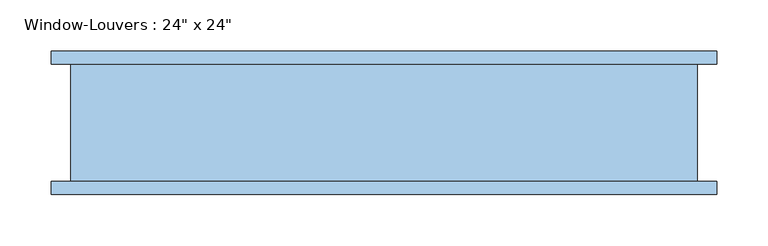
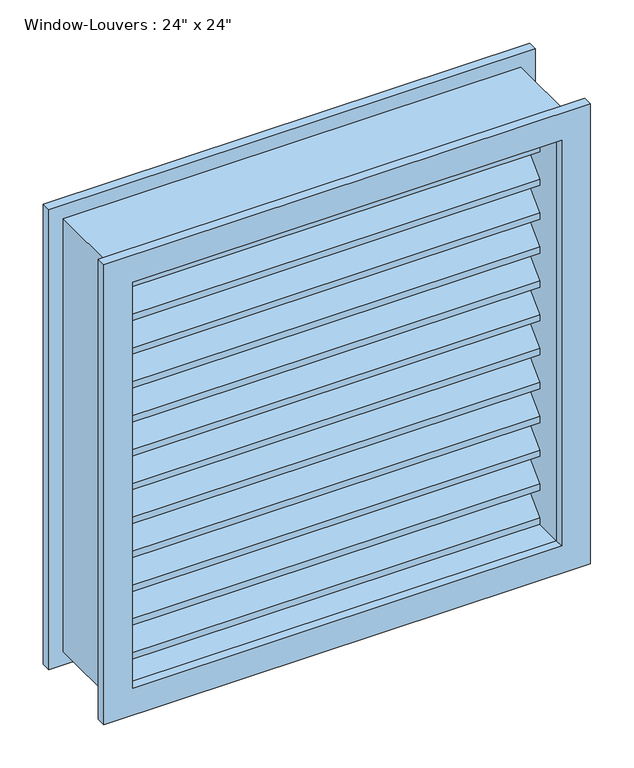
"""IFC4 building model written with IfcOpenShell, lengths in millimetres: window geometry."""

from ifc_helpers import new_model, si_unit, frame, origin, place, context, project, spatial, polyline, outline, extrude, source, transform, mapped, element, save


def window_d39e7ecb(model_context):
    return source(origin(), model_context, "Body", "SweptSolid", [
        extrude(outline(polyline([(50.8, 1419.1754778), (50.8, 1410.1952217), (12.7, 1448.2952217), (-25.4, 1410.1952217), (-25.4, 1419.1754778), (12.7, 1457.2754778), (50.8, 1419.1754778)])), frame((-285.75, 0.0, 0.0), z_axis=(1.0, 0.0, 0.0), x_axis=(0.0, 1.0, 0.0)), (0.0, 0.0, 1.0), 571.5),
        extrude(outline(polyline([(50.8, 1371.5009557), (50.8, 1362.5206995), (12.7, 1400.6206995), (-25.4, 1362.5206995), (-25.4, 1371.5009557), (12.7, 1409.6009557), (50.8, 1371.5009557)])), frame((-285.75, 0.0, 0.0), z_axis=(1.0, 0.0, 0.0), x_axis=(0.0, 1.0, 0.0)), (0.0, 0.0, 1.0), 571.5),
        extrude(outline(polyline([(50.8, 1323.8264335), (50.8, 1314.8461774), (12.7, 1352.9461774), (-25.4, 1314.8461774), (-25.4, 1323.8264335), (12.7, 1361.9264335), (50.8, 1323.8264335)])), frame((-285.75, 0.0, 0.0), z_axis=(1.0, 0.0, 0.0), x_axis=(0.0, 1.0, 0.0)), (0.0, 0.0, 1.0), 571.5),
        extrude(outline(polyline([(50.8, 1276.1519113), (50.8, 1267.1716552), (12.7, 1305.2716552), (-25.4, 1267.1716552), (-25.4, 1276.1519113), (12.7, 1314.2519113), (50.8, 1276.1519113)])), frame((-285.75, 0.0, 0.0), z_axis=(1.0, 0.0, 0.0), x_axis=(0.0, 1.0, 0.0)), (0.0, 0.0, 1.0), 571.5),
        extrude(outline(polyline([(50.8, 1228.4773891), (50.8, 1219.497133), (12.7, 1257.597133), (-25.4, 1219.497133), (-25.4, 1228.4773891), (12.7, 1266.5773891), (50.8, 1228.4773891)])), frame((-285.75, 0.0, 0.0), z_axis=(1.0, 0.0, 0.0), x_axis=(0.0, 1.0, 0.0)), (0.0, 0.0, 1.0), 571.5),
        extrude(outline(polyline([(50.8, 1180.802867), (50.8, 1171.8226109), (12.7, 1209.9226109), (-25.4, 1171.8226109), (-25.4, 1180.802867), (12.7, 1218.902867), (50.8, 1180.802867)])), frame((-285.75, 0.0, 0.0), z_axis=(1.0, 0.0, 0.0), x_axis=(0.0, 1.0, 0.0)), (0.0, 0.0, 1.0), 571.5),
        extrude(outline(polyline([(50.8, 1133.1283448), (50.8, 1124.1480887), (12.7, 1162.2480887), (-25.4, 1124.1480887), (-25.4, 1133.1283448), (12.7, 1171.2283448), (50.8, 1133.1283448)])), frame((-285.75, 0.0, 0.0), z_axis=(1.0, 0.0, 0.0), x_axis=(0.0, 1.0, 0.0)), (0.0, 0.0, 1.0), 571.5),
        extrude(outline(polyline([(50.8, 1085.4538226), (50.8, 1076.4735665), (12.7, 1114.5735665), (-25.4, 1076.4735665), (-25.4, 1085.4538226), (12.7, 1123.5538226), (50.8, 1085.4538226)])), frame((-285.75, 0.0, 0.0), z_axis=(1.0, 0.0, 0.0), x_axis=(0.0, 1.0, 0.0)), (0.0, 0.0, 1.0), 571.5),
        extrude(outline(polyline([(50.8, 1037.7793005), (50.8, 1028.7990443), (12.7, 1066.8990443), (-25.4, 1028.7990443), (-25.4, 1037.7793005), (12.7, 1075.8793005), (50.8, 1037.7793005)])), frame((-285.75, 0.0, 0.0), z_axis=(1.0, 0.0, 0.0), x_axis=(0.0, 1.0, 0.0)), (0.0, 0.0, 1.0), 571.5),
        extrude(outline(polyline([(50.8, 990.1047783), (50.8, 981.1245222), (12.7, 1019.2245222), (-25.4, 981.1245222), (-25.4, 990.1047783), (12.7, 1028.2047783), (50.8, 990.1047783)])), frame((-285.75, 0.0, 0.0), z_axis=(1.0, 0.0, 0.0), x_axis=(0.0, 1.0, 0.0)), (0.0, 0.0, 1.0), 571.5),
        extrude(outline(polyline([(50.8, 1466.85), (50.8, 1457.8697439), (12.7, 1495.9697439), (-25.4, 1457.8697439), (-25.4, 1466.85), (12.7, 1504.95), (50.8, 1466.85)])), frame((-285.75, 0.0, 0.0), z_axis=(1.0, 0.0, 0.0), x_axis=(0.0, 1.0, 0.0)), (0.0, 0.0, 1.0), 571.5),
        extrude(outline(polyline([(50.8, 942.4302561), (50.8, 933.45), (12.7, 971.55), (-25.4, 933.45), (-25.4, 942.4302561), (12.7, 980.5302561), (50.8, 942.4302561)])), frame((-285.75, 0.0, 0.0), z_axis=(1.0, 0.0, 0.0), x_axis=(0.0, 1.0, 0.0)), (0.0, 0.0, 1.0), 571.5),
        extrude(outline(polyline([(1524.0, 304.8), (1524.0, -304.8), (914.4, -304.8), (914.4, 304.8), (1524.0, 304.8)]), holes=[polyline([(1504.95, 285.75), (933.45, 285.75), (933.45, -285.75), (1504.95, -285.75), (1504.95, 285.75)])]), frame((0.0, -63.5, 0.0), z_axis=(0.0, 1.0, 0.0), x_axis=(0.0, 0.0, 1.0)), (0.0, 0.0, 1.0), 114.3),
        extrude(outline(polyline([(1543.05, 323.85), (1543.05, -323.85), (895.35, -323.85), (895.35, 323.85), (1543.05, 323.85)]), holes=[polyline([(1504.95, 285.75), (933.45, 285.75), (933.45, -285.75), (1504.95, -285.75), (1504.95, 285.75)])]), frame((0.0, -76.2, 0.0), z_axis=(0.0, 1.0, 0.0), x_axis=(0.0, 0.0, 1.0)), (0.0, 0.0, 1.0), 12.7),
        extrude(outline(polyline([(1543.05, -323.85), (895.35, -323.85), (895.35, 323.85), (1543.05, 323.85), (1543.05, -323.85)]), holes=[polyline([(1504.95, -285.75), (1504.95, 285.75), (933.45, 285.75), (933.45, -285.75), (1504.95, -285.75)])]), frame((0.0, 50.8, 0.0), z_axis=(0.0, 1.0, 0.0), x_axis=(0.0, 0.0, 1.0)), (0.0, 0.0, 1.0), 12.7),
    ])


if __name__ == "__main__":
    model = new_model("IFC4")
    model_context = context("Model", 3, world=origin())
    ifc_project = project(units=[si_unit("LENGTHUNIT", "METRE", prefix="MILLI")], contexts=[model_context])
    site = spatial("IfcSite", under=ifc_project)
    building = spatial("IfcBuilding", under=site)
    placement = place(None, origin())
    window_shape = window_d39e7ecb(model_context)
    element("IfcWindow", 1, ObjectType="Window-Louvers : 24\" x 24\"", at=placement, inside=building, context=model_context, shape_type="MappedRepresentation", body=[
        mapped(window_shape, transform((0.0, 0.0, 0.0), x_axis=(1.0, 0.0, 0.0), y_axis=(0.0, 1.0, 0.0), z_axis=(0.0, 0.0, 1.0))),
    ])
    save(model, "model.ifc")

# Revit data of these elements
# Type "Window-Louvers : 24\" x 24\""
#   Type Mark = "18"
#   Construction Type Id = "GSP4R"
#   Assembly Code = "B20"
#   Analytic Construction = "1/8 in Pilkington single glazing"
#   Visual Light Transmittance = 0.9
#   Thermal Resistance (R) = 1.53941 (h·ft²·°F)/BTU
#   Solar Heat Gain Coefficient = 0.78
#   Max Height = 1' - 11.74264"
#   Height = 2' - 0"
#   Heat Transfer Coefficient (U) = 0.6496 BTU/(h·ft²·°F)
#   Blade Width [instance default] = 1' - 10 1/2"
#   Blade Vertical Thickness = 0' - 0.35355"
#   Blade Thickness = 0' - 0 1/4"
#   Blade Spacing = 0' - 1 1/2"
#   Blade Height = 0' - 1.85355"
#   Blade Depth = 0' - 3"
#   Blade Angle = 45.00°
#   Default Sill Height = 3' - 0"
#   Trim Projection_Exterior = 0' - 0 1/2"
#   Trim Projection_Interior = 0' - 0 1/2"
#   Trim Width_Exterior = 0' - 1 1/2"
#   Trim Width_Interior = 0' - 1 1/2"
#   Width = 2' - 0"
#   Max Blade Count = 12
#   Define Thermal Properties by = 1
#   Blade Count = 12
#   Frame Material = Birch
#   Louver Material = Birch
#   Trim Exterior Material = Birch
#   Trim Interior Material = Birch
#   Wall Closure = (empty or 0)
# Element 1 (IfcWindow, "Window-Louvers : 24\" x 24\"")
#   Materials on its faces: "Birch"
# Materials
#   "Birch": class "Wood", colour RGB 224 178 126, transparency 0, Description = "Betula Alleghaniensis", Cost = 0
